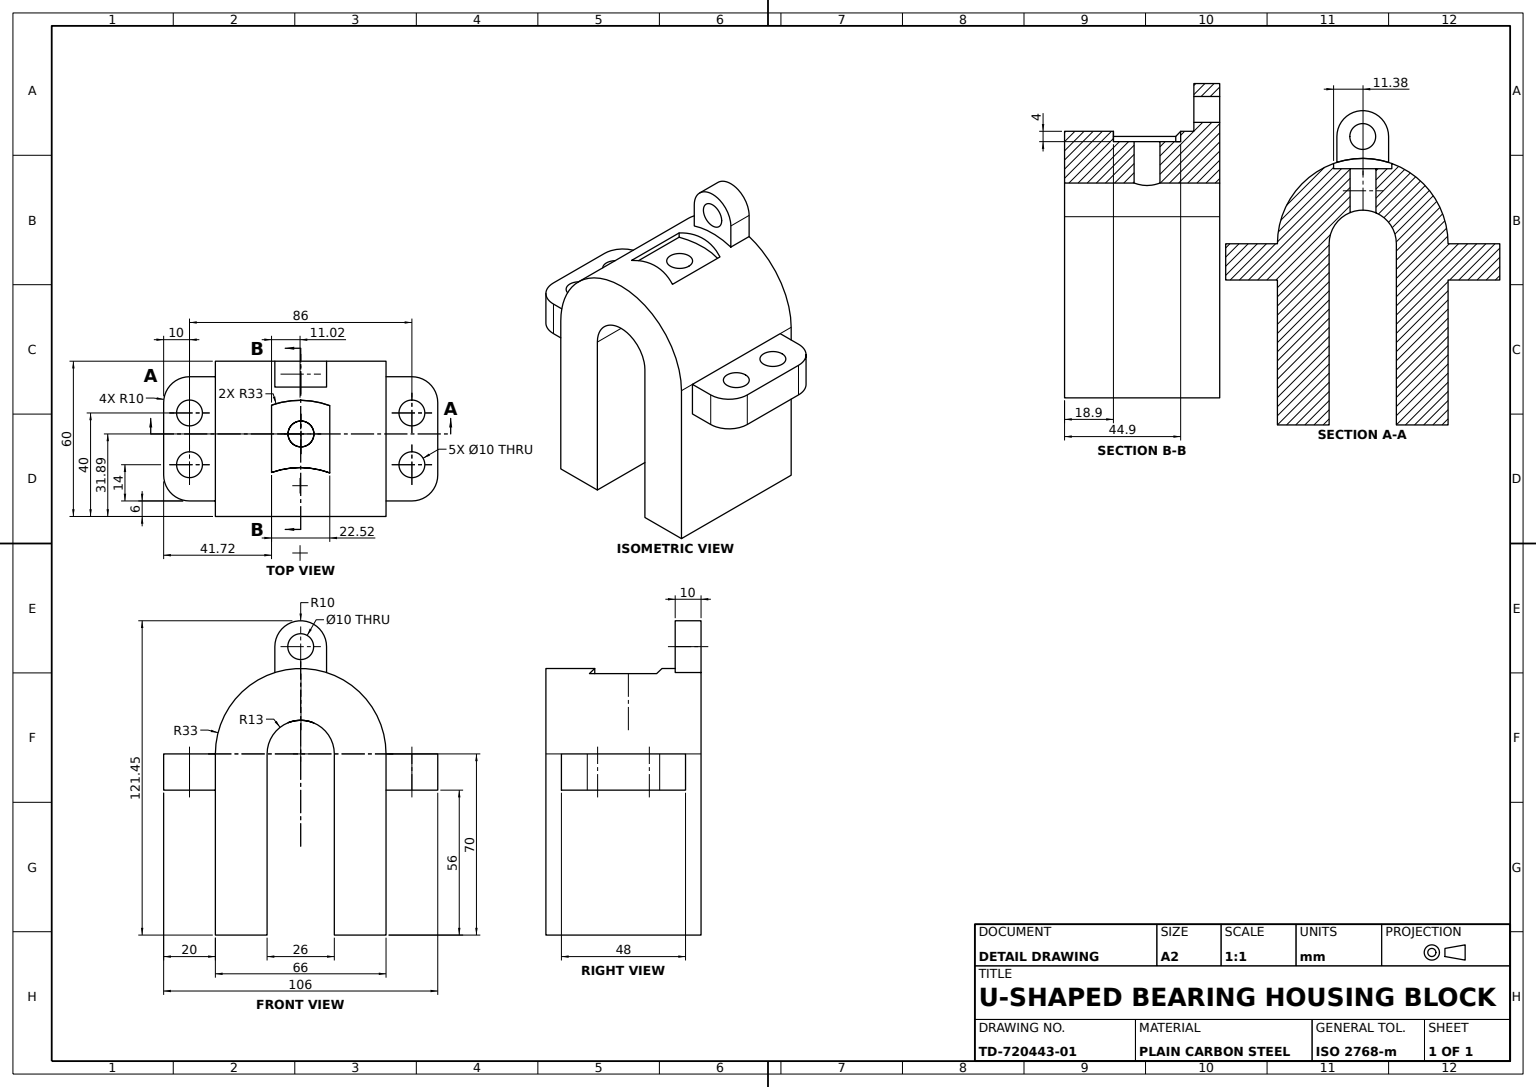
SolidWorks part; units mm, degrees
material "Plain Carbon Steel"
ref_plane "Front Plane" through (0, 0, 0) normal (0, 0, 1) x (1, 0, 0)
ref_plane "Top Plane" through (0, 0, 0) normal (0, 1, 0) x (1, 0, 0)
ref_plane "Right Plane" through (0, 0, 0) normal (1, 0, 0) x (0, 0, -1)
sketch "Body Profile Sketch" plane through (0, 0, 0) normal (0, 0, 1) x (1, 0, 0)
  line L0 (0, 0) -> (0, 70)
  line L1 (66, 70) -> (66, 0)
  line L3 (0, 0) -> (20, 0)
  line L4 (20, 0) -> (20, 70)
  line L5 (46, 70) -> (46, 0)
  line L6 (46, 0) -> (66, 0)
  arc A0 (0, 70) -> (66, 70) centre (33, 70) cw
  arc A1 (20, 70) -> (46, 70) centre (33, 70) cw
  dimension "D3" = 33
  dimension "D4" = 20
  dimension "D1" = 70
  dimension "D2" = 66
extrude "Housing Body 60" add sketch "Body Profile Sketch" against normal blind 60
sketch "Lifting Lug Sketch" plane through (0, 0, -60) normal (0, 0, -1) x (-1, 0, 0)
  line L0 (-43, 101.4484) -> (-43, 111.4484)
  line L1 (-23, 111.4484) -> (-23, 101.4484)
  arc A0 (0, 70) -> (-66, 70) centre (-33, 70) ccw construction
  arc A1 (-43, 111.4484) -> (-23, 111.4484) centre (-33, 111.4484) cw
  circle A2 centre (-33, 111.4484) radius 5
  arc A3 (-43, 101.4484) -> (-23, 101.4484) centre (-33, 70) cw
  point P9 (-33, 103)
  dimension "D1" = 10
  dimension "D3" = 10
  dimension "D4" = 33
  dimension "D2" = 10
extrude "Lifting Lug" add sketch "Lifting Lug Sketch" against normal blind 10
ref_plane "Flange Sketch Plane" through (0, 70, 0) normal (0, 1, 0) x (1, 0, 0)
sketch "Mounting Flanges Sketch" plane through (0, 70, 0) normal (0, 1, 0) x (1, 0, 0)
  line L2 (66, 54) -> (86, 54)
  line L3 (66, 54) -> (66, 6)
  line L4 (66, 6) -> (86, 6)
  line L5 (86, 54) -> (86, 6)
  line L6 (66, 60) -> (66, 0) construction
  line L7 (33, 50) -> (33, 0) construction
  line L8 (23, 50) -> (43, 50) construction
  line L9 (0, 0) -> (66, 0) construction
  line L10 (0, 6) -> (-20, 6)
  line L11 (-20, 54) -> (-20, 6)
  line L12 (0, 54) -> (-20, 54)
  line L13 (0, 54) -> (0, 6)
  circle A0 centre (76, 20) radius 5
  circle A1 centre (76, 40) radius 5
  circle A2 centre (-10, 40) radius 5
  circle A3 centre (-10, 20) radius 5
  point P6 (66, 30)
  point P7 (66, 30)
  point P12 (76, 54)
  dimension "D3" = 10
  dimension "D1" = 48
  dimension "D2" = 20
  dimension "D4" = 20
  dimension "D5" = 14
extrude "Mounting Flanges 14" add sketch "Mounting Flanges Sketch" against normal blind 14
fillet "Flange Corner Fillet R10 A" radius 10 1 edges at (86, 63, -54)
fillet "Flange Corner Fillet R10 B" radius 10 1 edges at (86, 63, -6)
fillet "Flange Corner Fillet R10 C" radius 10 1 edges at (-20, 63, -54)
fillet "Flange Corner Fillet R10 D" radius 10 1 edges at (-20, 63, -6)
ref_plane "Top Recess Plane" through (0, 103, 0) normal (0, 1, 0) x (1, 0, 0)
sketch "Top Recess Sketch" plane through (0, 103, 0) normal (0, 1, 0) x (1, 0, 0)
  line L0 (21.7248, 43) -> (21.7248, 17)
  line L1 (44.245, 42.8283) -> (44.245, 16.8283)
  line L2 (33, 60) -> (33, 0) construction
  line L3 (66, 54) -> (66, 6) construction
  arc A0 (21.7248, 43) -> (44.245, 42.8283) centre (32.7485, 11.8957) cw
  arc A1 (21.7248, 17) -> (44.245, 16.8283) centre (32.7485, -14.1043) cw
  point P8 (33, 44.8947)
  point P11 (66, 30)
  point P12 (21.7248, 30)
  dimension "D2" = 33
  dimension "D3" = 33
  dimension "D1" = 26
  dimension "D4" = 11.0237
  dimension "D5" = 11.2752
extrude "Top Recess 4 Deep" cut sketch "Top Recess Sketch" against normal blind 4
sketch "Recess Hole Sketch" plane through (0, 99, 0) normal (0, 1, 0) x (1, 0, 0)
  line L0 (21.7248, 43) -> (21.7248, 17) construction
  circle A0 centre (33.1089, 31.8924) radius 5
  arc A2 (44.245, 42.8283) -> (21.7248, 43) centre (32.7485, 11.8957) ccw construction
  dimension "D1" = 10
  dimension "D2" = 20
  dimension "D3" = 11.3841
extrude "Recess Hole" cut sketch "Recess Hole Sketch" against normal through all
